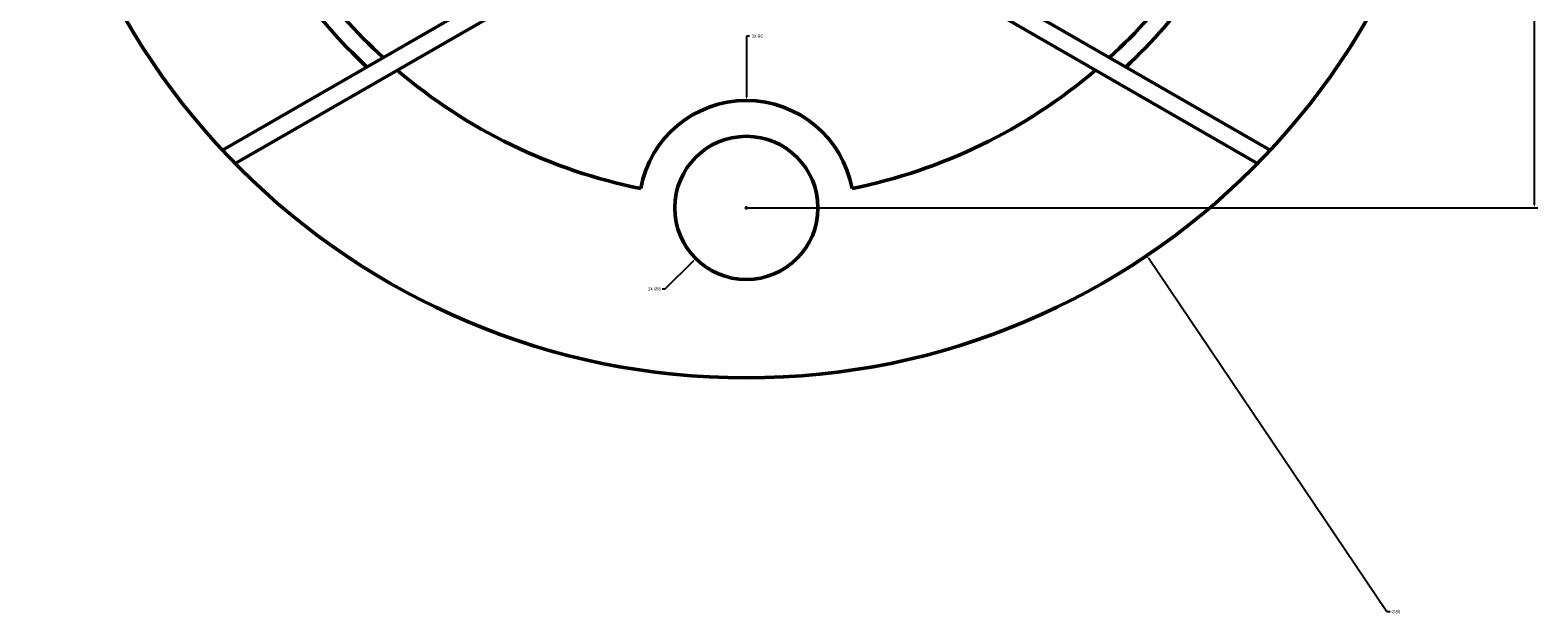
# Model space of a CAD drawing. Units: inches. Extents: x -19.9 to 72.3, y -39.8 to 57.5.
# Tile 1 of 8: x -11.9 to 72.3, y -39.8 to -7.2. Entities that reach past the tile are written whole.
import ezdxf

# ---------------------------------------------------------------- set-up
doc = ezdxf.new("R2010")
doc.units = ezdxf.units.IN
doc.header["$MEASUREMENT"] = 0
for name, color, linetype, lineweight in [('M-DIMS', 2, 'Continuous', 18), ('M-OUTL', 7, 'Continuous', 50), ('M-OUTL-HOLE', 7, 'Continuous', 50), ('M-OUTL-SLOT', 7, 'Continuous', 50)]:
    doc.layers.add(name, color=color, linetype=linetype, lineweight=lineweight)
doc.styles.get("Standard").update_dxf_attribs({"font": 'arial.ttf'})
doc.dimstyles.get("Standard").update_dxf_attribs({"dimtxt": 0.18, "dimasz": 0.18, "dimexe": 0.18, "dimexo": 0.0625, "dimgap": 0.09, "dimtad": 0, "dimtih": 1, "dimtoh": 1, "dimdec": 4, "dimzin": 0, "dimdsep": 46, "dimtxsty": 'Standard', "dimcen": 0.09, "dimadec": 0, "dimazin": 0, "dimtfac": 1, "dimtdec": 4, "dimtofl": 0, "dimtmove": 0, "dimatfit": 3, "dimfxl": 1, "dimtolj": 1, "dimtzin": 0, "dimarcsym": 0})

# ---------------------------------------------------------------- blocks, each defined once
blk = doc.blocks.new('FLANGE-MOUNT-D8-RELIEVED')
blk.add_circle((0, 0), 4)
for centre, radius, start, end in [((26.414, -15.25), 30, 109.47122, 138.65617), ((0, 0), 6, 250.42865, 49.57135), ((26.414, -15.25), 30, 161.34383, 190.52878)]:
    blk.add_arc(centre, radius, start, end)
blk = doc.blocks.new('FLANGE-STRAIGHT-SLOT')
for p, q in [((0, 0), (0, 21.114)), ((1, -0.54), (1, 20.869))]:
    blk.add_line(p, q)
blk = doc.blocks.new('FLANGE-INTERRUPTED-ARC-SLOT')
for radius, start, end in [(30, 192.5424, 204.39482), (31, 193.12273, 204.48604), (30, 215.60518, 227.4576), (31, 215.51396, 226.87727)]:
    blk.add_arc((26.414, 15.25), radius, start, end)
blk = doc.blocks.new('*D6')
at = {"layer": 'Defpoints', "color": 0, "transparency": 16777216}
for p in [(28.06, 43.841), (28.06, -17.159), (72.086, -17.159)]:
    blk.add_point(p, dxfattribs=at)
at = {"layer": 'M-DIMS', "color": 0, "lineweight": -2, "transparency": 16777216}
for p, q in [((28.122, 43.841), (72.266, 43.841)), ((72.086, 43.661), (72.086, 13.523)), ((72.086, -16.979), (72.086, 13.159)), ((28.122, -17.159), (72.266, -17.159))]:
    blk.add_line(p, q, dxfattribs=at)
at = {"layer": 'M-DIMS', "color": 0, "transparency": 16777216}
for points in [[(72.056, 43.661), (72.116, 43.661), (72.086, 43.841)], [(72.056, -16.979), (72.116, -16.979), (72.086, -17.159)]]:
    blk.add_solid(points, dxfattribs=at)
at = {"layer": 'M-DIMS', "color": 0, "transparency": 16777216, "insert": (72.086, 13.341), "char_height": 0.18, "attachment_point": 5}
blk.add_mtext('\\A1;61', dxfattribs=at)
blk = doc.blocks.new('*D11')
at = {"layer": 'Defpoints', "color": 0, "transparency": 16777216}
for p in [(5.703, 46.51), (50.417, -19.828)]:
    blk.add_point(p, dxfattribs=at)
at = {"layer": 'M-DIMS', "color": 0, "lineweight": -2, "transparency": 16777216}
for p, q in [((27.97, 13.341), (28.15, 13.341)), ((28.06, 13.251), (28.06, 13.431)), ((63.831, -39.729), (50.517, -19.977)), ((64.011, -39.729), (63.831, -39.729))]:
    blk.add_line(p, q, dxfattribs=at)
at = {"layer": 'M-DIMS', "color": 0, "transparency": 16777216}
blk.add_solid([(50.542, -19.96), (50.492, -19.994), (50.417, -19.828)], dxfattribs=at)
at = {"layer": 'M-DIMS', "color": 0, "transparency": 16777216, "insert": (64.327, -39.729), "char_height": 0.18, "attachment_point": 5}
blk.add_mtext('\\A1;∅80', dxfattribs=at)
blk = doc.blocks.new('*D17')
at = {"layer": 'Defpoints', "color": 0, "transparency": 16777216}
for p in [(28.06, -11.159), (28.06, -17.159)]:
    blk.add_point(p, dxfattribs=at)
at = {"layer": 'M-DIMS', "color": 0, "lineweight": -2, "transparency": 16777216}
for p, q in [((28.24, -7.559), (28.06, -7.559)), ((28.06, -7.559), (28.06, -10.979)), ((27.97, -17.159), (28.15, -17.159)), ((28.06, -17.249), (28.06, -17.069))]:
    blk.add_line(p, q, dxfattribs=at)
at = {"layer": 'M-DIMS', "color": 0, "transparency": 16777216}
blk.add_solid([(28.03, -10.979), (28.09, -10.979), (28.06, -11.159)], dxfattribs=at)
at = {"layer": 'M-DIMS', "color": 0, "transparency": 16777216, "insert": (28.668, -7.559), "char_height": 0.18, "attachment_point": 5}
blk.add_mtext('\\A1;3X R6', dxfattribs=at)
blk = doc.blocks.new('*D20')
at = {"layer": 'Defpoints', "color": 0, "transparency": 16777216}
for p in [(30.888, -14.33), (25.232, -19.987)]:
    blk.add_point(p, dxfattribs=at)
at = {"layer": 'M-DIMS', "color": 0, "lineweight": -2, "transparency": 16777216}
for p, q in [((27.97, -17.159), (28.15, -17.159)), ((28.06, -17.249), (28.06, -17.069)), ((23.535, -21.684), (25.104, -20.115)), ((23.355, -21.684), (23.535, -21.684))]:
    blk.add_line(p, q, dxfattribs=at)
at = {"layer": 'M-DIMS', "color": 0, "transparency": 16777216}
blk.add_solid([(25.083, -20.093), (25.126, -20.136), (25.232, -19.987)], dxfattribs=at)
at = {"layer": 'M-DIMS', "color": 0, "transparency": 16777216, "insert": (22.919, -21.684), "char_height": 0.18, "attachment_point": 5}
blk.add_mtext('\\A1;3X ∅8', dxfattribs=at)

msp = doc.modelspace()

# ---------------------------------------------------------------- linework, layer by layer
at = {"layer": 'M-OUTL'}
msp.add_circle((28.06, 13.341), 40, dxfattribs=at)

# ---------------------------------------------------------------- block references
at = {"layer": 'M-OUTL-HOLE', "rotation": 120}
msp.add_blockref('FLANGE-MOUNT-D8-RELIEVED', (28.06, -17.159), dxfattribs=at)
at = {"layer": 'M-OUTL-SLOT'}
msp.add_blockref('FLANGE-INTERRUPTED-ARC-SLOT', (1.646, -1.909), dxfattribs=at)
for name, p, rotation in [('FLANGE-INTERRUPTED-ARC-SLOT', (54.474, -1.909), 120), ('FLANGE-STRAIGHT-SLOT', (39.028, -3.383), 240)]:
    msp.add_blockref(name, p, dxfattribs=dict(at, rotation=rotation))
at = {"layer": 'M-OUTL-SLOT', "extrusion": (0, 0, -1), "zscale": -1, "rotation": 239.9999999999999}
msp.add_blockref('FLANGE-STRAIGHT-SLOT', (-17.092, -3.383), dxfattribs=at)

# ---------------------------------------------------------------- dimensions: what is measured, and where the dimension line sits
at = {"layer": 'M-DIMS'}
dim = msp.add_diameter_dim_2p(p1=(5.703, 46.51), p2=(50.417, -19.828), dimstyle='Standard', override={"dimdec": 0, "dimlfac": 1, "dimrnd": 0, "dimzin": 0, "dimdsep": 46, "dimlunit": 2}, dxfattribs=at)
dim.commit()
dim.dimension.update_dxf_attribs({"geometry": '*D11', "text_midpoint": (64.327, -39.729), "dimtype": 163})
dim = msp.add_linear_dim(base=(72.086, -17.159), p1=(28.06, 43.841), p2=(28.06, -17.159), angle=90, dimstyle='Standard', override={"dimdec": 0, "dimlfac": 1, "dimrnd": 0, "dimzin": 0, "dimdsep": 46, "dimlunit": 2}, dxfattribs=at)
dim.commit()
dim.dimension.update_dxf_attribs({"geometry": '*D6', "text_midpoint": (72.086, 13.341)})
dim = msp.add_radius_dim(center=(28.06, -17.159), mpoint=(28.06, -11.159), text='3X <>', dimstyle='Standard', override={"dimdec": 0, "dimlfac": 1, "dimrnd": 0, "dimzin": 0, "dimdsep": 46, "dimlunit": 2}, dxfattribs=at)
dim.commit()
dim.dimension.update_dxf_attribs({"geometry": '*D17', "text_midpoint": (28.668, -7.559), "dimtype": 164})
dim = msp.add_diameter_dim_2p(p1=(30.888, -14.33), p2=(25.232, -19.987), text='3X <>', dimstyle='Standard', override={"dimdec": 0, "dimlfac": 1, "dimrnd": 0, "dimzin": 0, "dimdsep": 46, "dimlunit": 2}, dxfattribs=at)
dim.commit()
dim.dimension.update_dxf_attribs({"geometry": '*D20', "text_midpoint": (22.919, -21.684), "dimtype": 163})

doc.saveas('drawing.dxf')
